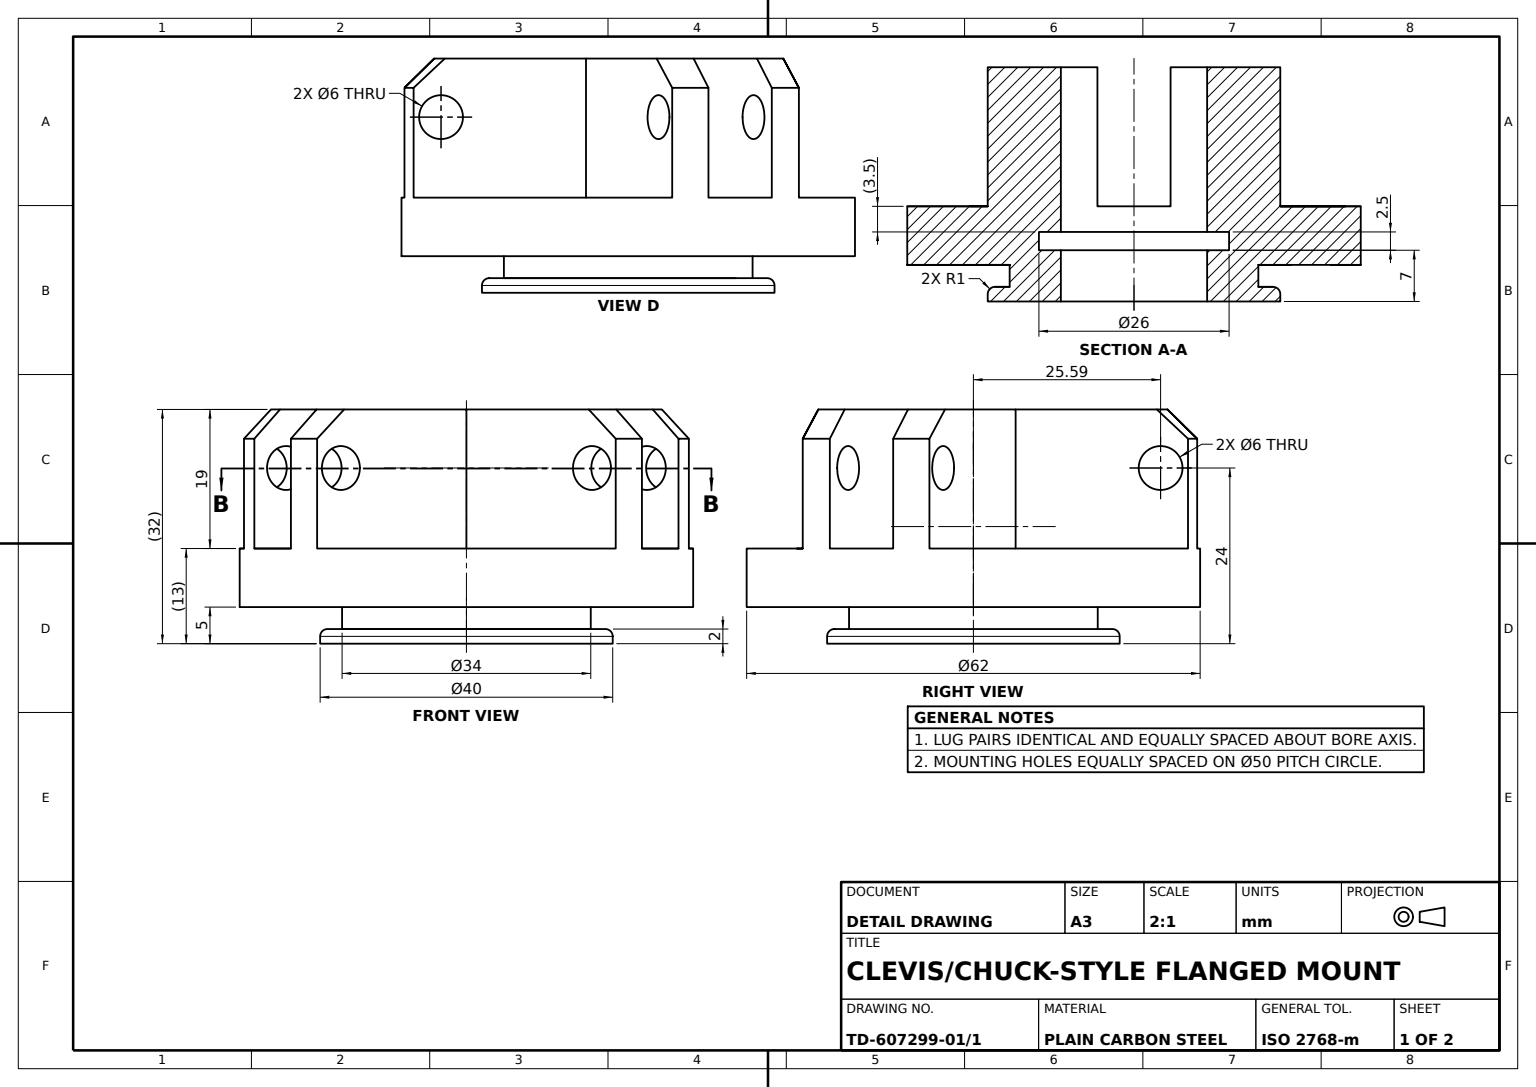
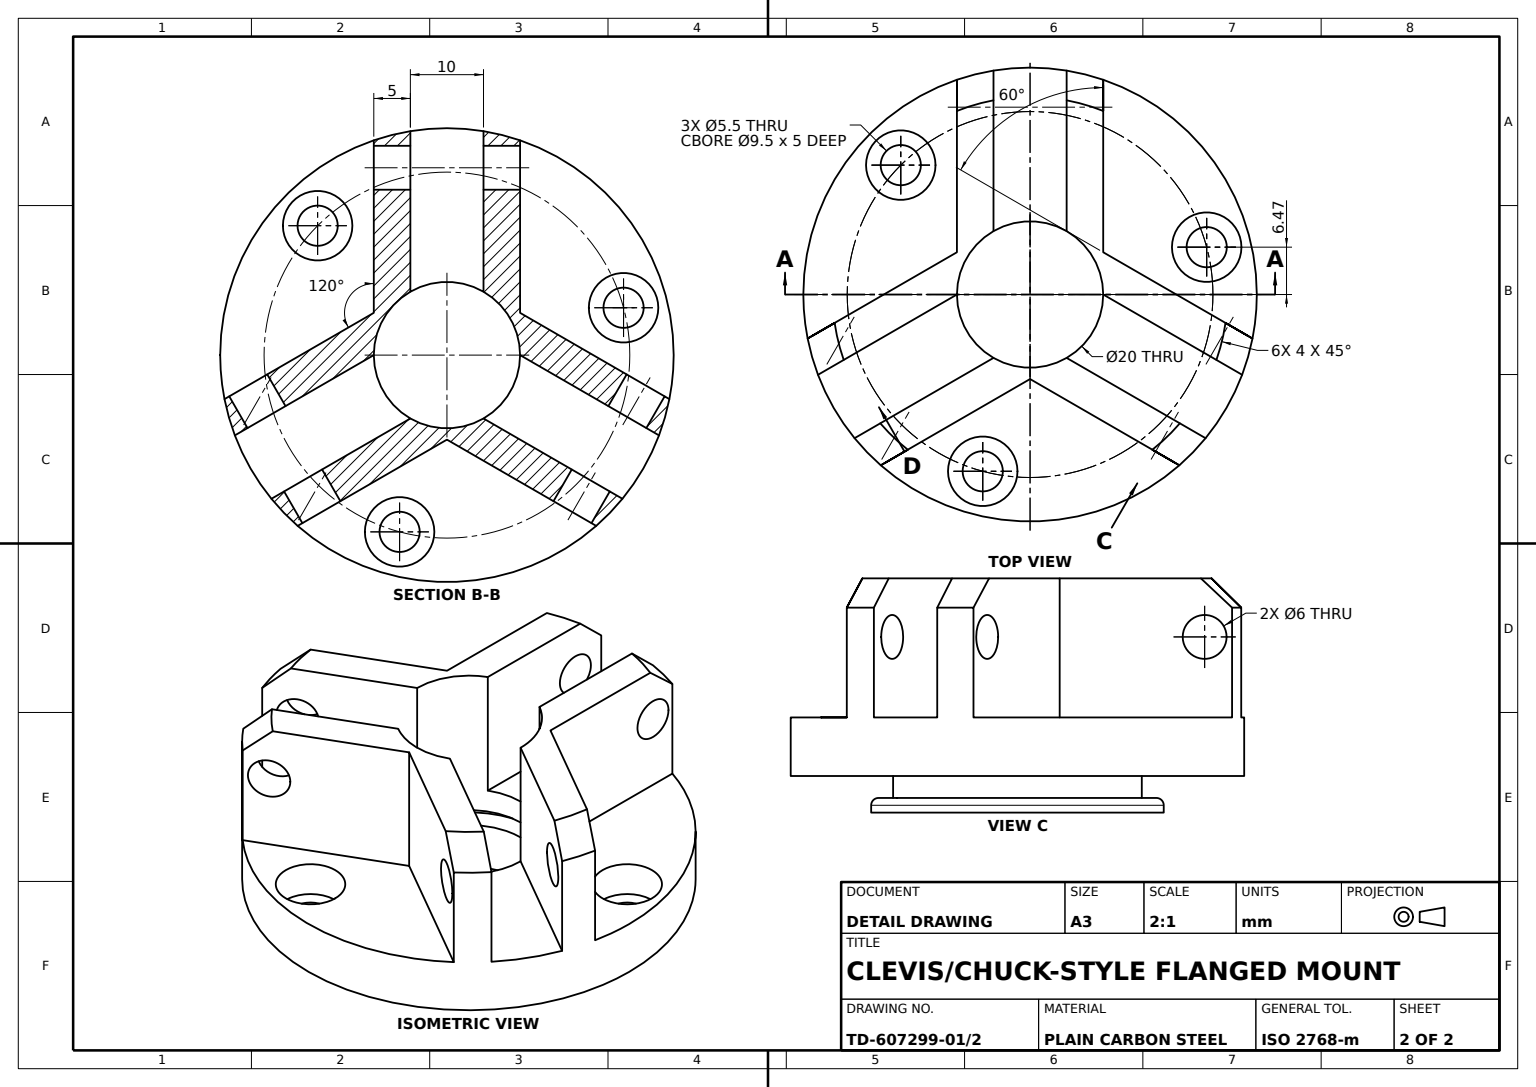
from build123d import *
from build123d.topology import SkipClean

# Parameters (mm, degrees)
LUG_DEPTH                         = 19
LUG_PIN_HOLE_A_SKETCH_R           = 3
LUG_PIN_HOLE_A_6_DEPTH            = 19
LUG_PIN_HOLE_B_SKETCH_R           = 3
LUG_PIN_HOLE_B_6_DEPTH            = 19
LUG_PATTERN_3X120_COUNT           = 3
LUG_CHAMFER_4MM_SIZE              = 4
BORE_START                        = -3.5
BORE_RECESS_SKETCH_R              = 10
BORE_RECESS_20_X3_5_DEPTH         = 3.5
CENTRE_BORE_SKETCH_R              = 10
CENTRE_BORE_20_X7_DEPTH           = 7
COUNTERBORE_SKETCH_R              = 13
COUNTERBORE_26_X2_5_DEPTH         = 2.5
RADIAL_SLOT_PROFILE_R             = 4.75
RADIAL_SLOT_DEPTH                 = 5
FLANGE_HOLE_SKETCH_R              = 2.75
FLANGE_HOLE_5_5_DEPTH             = 50.979995998
SLOT_AND_HOLE_PATTERN_3X120_COUNT = 3


with BuildPart() as part:
    # Base Flange Profile → Base Flange Ø62 (revolve)
    with BuildSketch(Plane.XY):
        with BuildLine():
            Line((-31, 4), (-31, -4))
            Line((-31, -4), (-17, -4))
            Line((-17, -4), (-17, -7))
            Line((-17, -7), (-19, -7))
            ThreePointArc((-19, -7), (-19.707106781, -7.292893219), (-20, -8))
            Line((-20, -8), (-20, -9))
            Line((-20, -9), (0, -9))
            Line((0, -9), (0, 4))
            Line((0, 4), (-31, 4))
        make_face()
    revolve(axis=Axis((0, 39.539668131, 0), (0, -1, 0)))

    # Lug Profile → Lug (add)
    with SkipClean():  # the faces are left unmerged after this step: merging them gives an invalid solid
        with BuildSketch(Plane(origin=(0, 4, 0), x_dir=(1, 0, 0), z_dir=(0, 1, 0))):
            with BuildLine():
                Line((5, 30.594117082), (5, 8.660254038))
                ThreePointArc((5, 8.660254038), (8.660254038, 5), (10, 0))
                Line((10, 0), (28.995282599, -10.966931522))
                ThreePointArc((28.995282599, -10.966931522), (29.806622049, -8.518525814), (30.411611519, -6.011146713))
                Line((30.411611519, -6.011146713), (10, 5.773502692))
                Line((10, 5.773502692), (10, 29.342801502))
                ThreePointArc((10, 29.342801502), (7.526051267, 30.072554802), (5, 30.594117082))
            make_face()
        lug = extrude(amount=LUG_DEPTH)

    # Lug Pin Hole A Sketch → Lug Pin Hole A Ø6 (cut)
    with SkipClean():  # the faces are left unmerged after this step: merging them gives an invalid solid
        with BuildSketch(Plane.ZY.offset(-5)):
            with Locations((-25.594117082, 15)):
                Circle(LUG_PIN_HOLE_A_SKETCH_R)
        lug_pin_hole_a_6 = extrude(amount=-LUG_PIN_HOLE_A_6_DEPTH, mode=Mode.SUBTRACT)

    # Lug Pin Hole B Sketch → Lug Pin Hole B Ø6 (cut)
    with SkipClean():  # the faces are left unmerged after this step: merging them gives an invalid solid
        with BuildSketch(Plane(origin=(2.5, 0, -4.330127019), x_dir=(0.8660254037844399, 0, 0.4999999999999978), z_dir=(-0.4999999999999978, 0, 0.8660254037844399))):
            with Locations((25.594117082, 15)):
                Circle(LUG_PIN_HOLE_B_SKETCH_R)
        lug_pin_hole_b_6 = extrude(amount=-LUG_PIN_HOLE_B_6_DEPTH, mode=Mode.SUBTRACT)

    # Lug Pattern 3x120°: Lug, Lug Pin Hole A Ø6, Lug Pin Hole B Ø6 ×3 about axis
    with SkipClean():  # the faces are left unmerged after this step: merging them gives an invalid solid
        lug_pattern_3x120_axis = Axis((0, 0, 0), (0, 1, 0))
        add([lug.rotate(lug_pattern_3x120_axis, i * 360 / LUG_PATTERN_3X120_COUNT) for i in range(1, LUG_PATTERN_3X120_COUNT)])
        add([lug_pin_hole_a_6.rotate(lug_pattern_3x120_axis, i * 360 / LUG_PATTERN_3X120_COUNT) for i in range(1, LUG_PATTERN_3X120_COUNT)], mode=Mode.SUBTRACT)
        add([lug_pin_hole_b_6.rotate(lug_pattern_3x120_axis, i * 360 / LUG_PATTERN_3X120_COUNT) for i in range(1, LUG_PATTERN_3X120_COUNT)], mode=Mode.SUBTRACT)

    # Lug Chamfer 4mm
    lug_chamfer_4mm_edges = [part.edges().sort_by_distance(p)[0] for p in [
        (29.806622049, 23, 8.518525814),
        (7.526051267, 23, -30.072554802),
        (-7.526051267, 23, -30.072554802),
        (-29.806622049, 23, 8.518525814),
        (-22.280570782, 23, 21.554028988),
        (22.280570782, 23, 21.554028988),
    ]]
    chamfer(lug_chamfer_4mm_edges, length=LUG_CHAMFER_4MM_SIZE)

    # Bore Recess Sketch → Bore Recess Ø20 x3.5 (cut)
    with BuildSketch(Plane(origin=(0, 4, 0), x_dir=(1, 0, 0), z_dir=(0, 1, 0)).offset(BORE_START)):
        with Locations(Location((0, 0, 0), (0, 0, 180))):
            Circle(BORE_RECESS_SKETCH_R)
    extrude(amount=BORE_RECESS_20_X3_5_DEPTH, mode=Mode.SUBTRACT)

    # Centre Bore Sketch → Centre Bore Ø20 x7 (cut)
    with BuildSketch(Plane.XZ.offset(9)):
        with Locations(Location((0, 0, 0), (0, 0, 180))):
            Circle(CENTRE_BORE_SKETCH_R)
    extrude(amount=-CENTRE_BORE_20_X7_DEPTH, mode=Mode.SUBTRACT)

    # Counterbore Sketch → Counterbore Ø26 x2.5 (cut)
    with BuildSketch(Plane.XZ.offset(2)):
        Circle(COUNTERBORE_SKETCH_R)
    extrude(amount=-COUNTERBORE_26_X2_5_DEPTH, mode=Mode.SUBTRACT)

    # Radial Slot Profile → Radial Slot (cut)
    with BuildSketch(Plane(origin=(0, 4, 0), x_dir=(1, 0, 0), z_dir=(0, 1, 0))):
        with Locations(Location((-6.470476128, -24.148145657, 0), (0, 0, 180))):
            Circle(RADIAL_SLOT_PROFILE_R)
    radial_slot = extrude(amount=-RADIAL_SLOT_DEPTH, mode=Mode.SUBTRACT)

    # Flange Hole Sketch → Flange Hole Ø5.5 (cut, through all)
    with BuildSketch(Plane(origin=(0, -1, 0), x_dir=(1, 0, 0), z_dir=(0, 1, 0))):
        with Locations(Location((-6.470476128, -24.148145657, 0), (0, 0, 180))):
            Circle(FLANGE_HOLE_SKETCH_R)
    flange_hole_5_5 = extrude(amount=-FLANGE_HOLE_5_5_DEPTH, mode=Mode.SUBTRACT)

    # Slot and Hole Pattern 3x120°: Radial Slot, Flange Hole Ø5.5 ×3 about axis
    slot_and_hole_pattern_3x120_axis = Axis((0, 0, 0), (0, 1, 0))
    add([radial_slot.rotate(slot_and_hole_pattern_3x120_axis, i * 360 / SLOT_AND_HOLE_PATTERN_3X120_COUNT) for i in range(1, SLOT_AND_HOLE_PATTERN_3X120_COUNT)], mode=Mode.SUBTRACT)
    add([flange_hole_5_5.rotate(slot_and_hole_pattern_3x120_axis, i * 360 / SLOT_AND_HOLE_PATTERN_3X120_COUNT) for i in range(1, SLOT_AND_HOLE_PATTERN_3X120_COUNT)], mode=Mode.SUBTRACT)


solid = part.part
